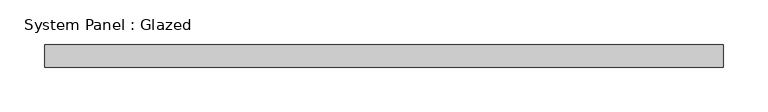
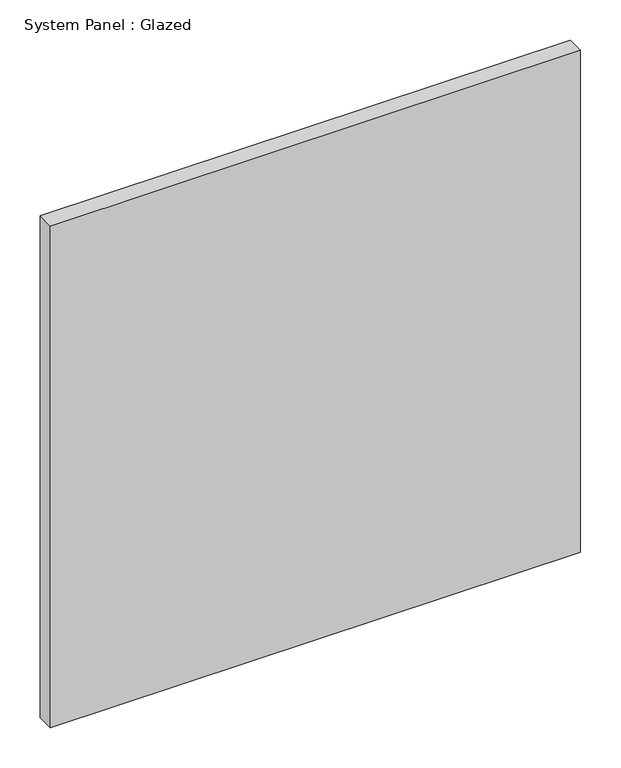
"""IFC4 building model written with IfcOpenShell, lengths in millimetres: plate geometry, System Panel : Glazed."""

from ifc_helpers import new_model, si_unit, origin, origin_with_axes, place, context, project, spatial, polyline, outline, extrude, source, transform, mapped, element, save


def system_panel_glazed_550407b1(model_context):
    return source(origin(), model_context, "Body", "SweptSolid", [
        extrude(outline(polyline([(381.0, 19.05), (-381.0, 19.05), (-381.0, 44.45), (381.0, 44.45), (381.0, 19.05)])), origin_with_axes(), (0.0, 0.0, 1.0), 762.0),
    ])


if __name__ == "__main__":
    model = new_model("IFC4")
    model_context = context("Model", 3, world=origin())
    ifc_project = project(units=[si_unit("LENGTHUNIT", "METRE", prefix="MILLI")], contexts=[model_context])
    site = spatial("IfcSite", under=ifc_project)
    building = spatial("IfcBuilding", under=site)
    placement = place(None, origin())
    system_panel_glazed_shape = system_panel_glazed_550407b1(model_context)
    element("IfcPlate", 1, ObjectType="System Panel : Glazed", at=placement, inside=building, context=model_context, shape_type="MappedRepresentation", body=[
        mapped(system_panel_glazed_shape, transform((0.0, 0.0, 0.0), x_axis=(1.0, 0.0, 0.0), y_axis=(0.0, 1.0, 0.0), z_axis=(0.0, 0.0, 1.0))),
    ])
    save(model, "model.ifc")

# Revit data of these elements
# Type "System Panel : Glazed"
#   Construction Type Id = "GSP4R"
#   Analytic Construction = "1/8 in Pilkington single glazing"
#   Visual Light Transmittance = 0.9
#   Solar Heat Gain Coefficient = 0.86
#   Heat Transfer Coefficient (U) = 1.18115 BTU/(h·ft²·°F)
# Element 1 (IfcPlate, "System Panel : Glazed")
#   Materials on its faces: "Glass"
# Materials
#   "Glass": class "Glass", colour RGB 0 128 192, transparency 0.75, Description = "Soda Lime Glass", Cost = 0
